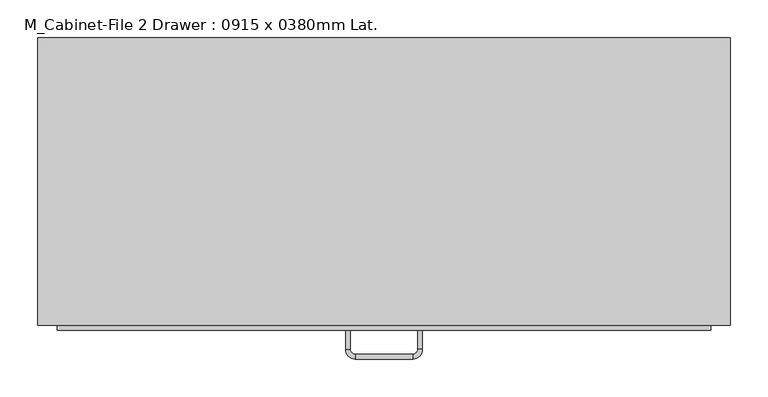
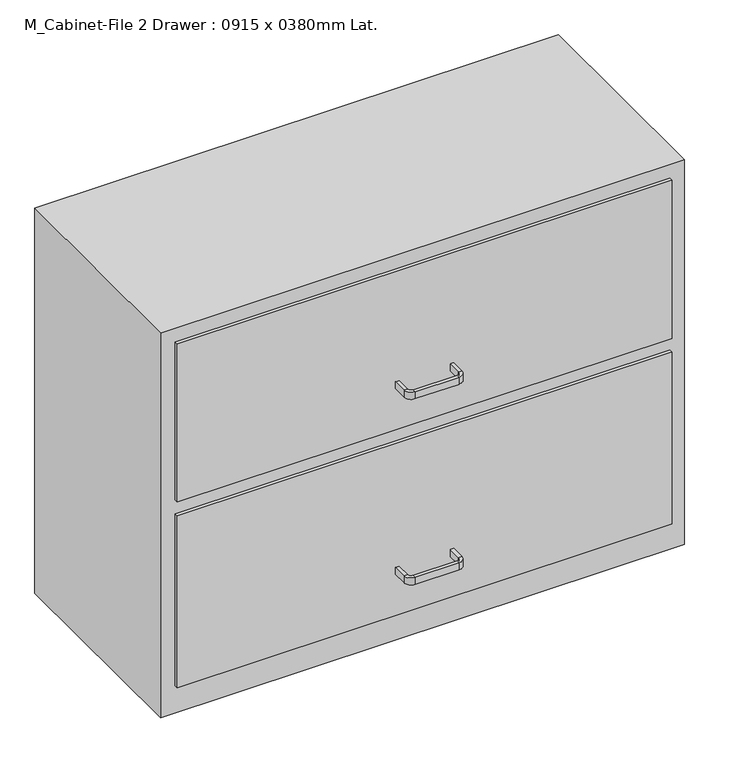
"""IFC4 building model written with IfcOpenShell, lengths in millimetres: furniture geometry, M_Cabinet-File 2 Drawer : 0915 x 0380mm Lat.."""

from ifc_helpers import new_model, si_unit, frame, origin, origin_with_axes, place, context, project, spatial, polyline, circle_curve, outline, extrude, source, transform, mapped, element, save
from ifc_brep_helpers import plane_surface, cylinder_surface, revolved_surface, advanced_brep


def m_cabinet_file_2_drawer_0915_x_0380mm_lat_9df0d5dd(model_context):
    return source(origin(), model_context, "Body", "SolidModel", [
        extrude(outline(polyline([(304.203553, -338.4843001), (-559.996447, -338.4843001), (-559.996447, -332.1343001), (304.203553, -332.1343001), (304.203553, -338.4843001)])), frame((0.0, 0.0, 393.7), z_axis=(0.0, 0.0, 1.0), x_axis=(1.0, 0.0, 0.0)), (0.0, 0.0, 1.0), 291.9),
        extrude(outline(polyline([(304.203553, -338.4843001), (-559.996447, -338.4843001), (-559.996447, -332.1343001), (304.203553, -332.1343001), (304.203553, -338.4843001)])), frame((0.0, 0.0, 50.8), z_axis=(0.0, 0.0, 1.0), x_axis=(1.0, 0.0, 0.0)), (0.0, 0.0, 1.0), 317.5),
        advanced_brep(
        [(-172.346447, -338.4843001, 127.0), (-178.696447, -338.4843001, 127.0), (-178.696447, -338.4843001, 139.7), (-172.346447, -338.4843001, 139.7), (-172.346447, -363.8843001, 127.0), (-178.696447, -363.8843001, 127.0), (-178.696447, -363.8843001, 139.7), (-172.346447, -363.8843001, 139.7), (-165.996447, -376.5843001, 127.0), (-165.996447, -370.2343001, 127.0), (-165.996447, -376.5843001, 139.7), (-165.996447, -370.2343001, 139.7), (-89.796447, -370.2343001, 127.0), (-89.796447, -376.5843001, 127.0), (-89.796447, -376.5843001, 139.7), (-89.796447, -370.2343001, 139.7), (-77.096447, -363.8843001, 127.0), (-83.446447, -363.8843001, 127.0), (-77.096447, -363.8843001, 139.7), (-83.446447, -363.8843001, 139.7), (-83.446447, -338.4843001, 127.0), (-83.446447, -338.4843001, 139.7), (-77.096447, -338.4843001, 139.7), (-77.096447, -338.4843001, 127.0)],
        [
            (0, 1),
            (1, 2),
            (2, 3),
            (3, 0),
            (0, 4),
            (4, 5),
            (5, 1),
            (5, 6),
            (6, 2),
            (6, 7),
            (7, 3),
            (7, 4),
            (8, 5, circle_curve(frame((-165.996447, -363.8843001, 127.0), z_axis=(0.0, 0.0, -1.0), x_axis=(-1.0, 0.0, 0.0)), 12.7)),
            (4, 9, circle_curve(frame((-165.996447, -363.8843001, 127.0), z_axis=(0.0, 0.0, 1.0), x_axis=(-1.0, 0.0, 0.0)), 6.35)),
            (9, 8),
            (10, 6, circle_curve(frame((-165.996447, -363.8843001, 139.7), z_axis=(0.0, 0.0, -1.0), x_axis=(-1.0, 0.0, 0.0)), 12.7)),
            (8, 10),
            (11, 7, circle_curve(frame((-165.996447, -363.8843001, 139.7), z_axis=(0.0, 0.0, -1.0), x_axis=(-1.0, 0.0, 0.0)), 6.35)),
            (10, 11),
            (11, 9),
            (9, 12),
            (12, 13),
            (13, 8),
            (13, 14),
            (14, 10),
            (14, 15),
            (15, 11),
            (15, 12),
            (16, 13, circle_curve(frame((-89.796447, -363.8843001, 127.0), z_axis=(0.0, 0.0, -1.0), x_axis=(0.0, -1.0, 0.0)), 12.7)),
            (12, 17, circle_curve(frame((-89.796447, -363.8843001, 127.0), z_axis=(0.0, 0.0, 1.0), x_axis=(0.0, -1.0, 0.0)), 6.35)),
            (17, 16),
            (18, 14, circle_curve(frame((-89.796447, -363.8843001, 139.7), z_axis=(0.0, 0.0, -1.0), x_axis=(0.0, -1.0, 0.0)), 12.7)),
            (16, 18),
            (19, 15, circle_curve(frame((-89.796447, -363.8843001, 139.7), z_axis=(0.0, 0.0, -1.0), x_axis=(0.0, -1.0, 0.0)), 6.35)),
            (18, 19),
            (19, 17),
            (20, 21),
            (21, 22),
            (22, 23),
            (23, 20),
            (17, 20),
            (23, 16),
            (22, 18),
            (21, 19),
        ],
        [
            plane_surface(frame((-661.3382215, -338.4843001, 0.0), z_axis=(0.0, 1.0, 0.0), x_axis=(0.0, 0.0, -1.0))),
            plane_surface(frame((-172.346447, -338.4843001, 127.0), z_axis=(0.0, 0.0, -1.0), x_axis=(0.0, -1.0, 0.0))),
            plane_surface(frame((-178.696447, -338.4843001, 127.0), z_axis=(-1.0, 0.0, 0.0), x_axis=(0.0, -1.0, 0.0))),
            plane_surface(frame((-178.696447, -338.4843001, 139.7), z_axis=(0.0, 0.0, 1.0), x_axis=(0.0, -1.0, 0.0))),
            plane_surface(frame((-172.346447, -338.4843001, 139.7), z_axis=(1.0, 0.0, 0.0), x_axis=(0.0, -1.0, 0.0))),
            plane_surface(frame((-165.996447, -363.8843001, 127.0), z_axis=(0.0, 0.0, -1.0), x_axis=(-1.0, 0.0, 0.0))),
            cylinder_surface(frame((-165.996447, -363.8843001, 0.0), z_axis=(0.0, 0.0, 1.0), x_axis=(-1.0, 0.0, 0.0)), 12.7),
            plane_surface(frame((-165.996447, -363.8843001, 139.7), z_axis=(0.0, 0.0, 1.0), x_axis=(-1.0, 0.0, 0.0))),
            revolved_surface(polyline([(-172.34644699999998, -363.8843001, 139.7), (-172.34644699999998, -363.8843001, 127.0)]), (-165.996447, -363.8843001, 0.0), (0.0, 0.0, 1.0)),
            plane_surface(frame((-165.996447, -370.2343001, 127.0), z_axis=(0.0, 0.0, -1.0), x_axis=(1.0, 0.0, 0.0))),
            plane_surface(frame((-165.996447, -376.5843001, 127.0), z_axis=(0.0, -1.0, 0.0), x_axis=(1.0, 0.0, 0.0))),
            plane_surface(frame((-165.996447, -376.5843001, 139.7), z_axis=(0.0, 0.0, 1.0), x_axis=(1.0, 0.0, 0.0))),
            plane_surface(frame((-165.996447, -370.2343001, 139.7), z_axis=(0.0, 1.0, 0.0), x_axis=(1.0, 0.0, 0.0))),
            plane_surface(frame((-89.796447, -363.8843001, 127.0), z_axis=(0.0, 0.0, -1.0), x_axis=(0.0, -1.0, 0.0))),
            cylinder_surface(frame((-89.796447, -363.8843001, 0.0), z_axis=(0.0, 0.0, 1.0), x_axis=(0.0, -1.0, 0.0)), 12.7),
            plane_surface(frame((-89.796447, -363.8843001, 139.7), z_axis=(0.0, 0.0, 1.0), x_axis=(0.0, -1.0, 0.0))),
            revolved_surface(polyline([(-89.796447, -370.23430010000004, 139.7), (-89.796447, -370.23430010000004, 127.0)]), (-89.796447, -363.8843001, 0.0), (0.0, 0.0, 1.0)),
            plane_surface(frame((-559.7382215, -338.4843001, 0.0), z_axis=(0.0, 1.0, 0.0), x_axis=(0.0, 0.0, 1.0))),
            plane_surface(frame((-83.446447, -363.8843001, 127.0), z_axis=(0.0, 0.0, -1.0), x_axis=(0.0, 1.0, 0.0))),
            plane_surface(frame((-77.096447, -363.8843001, 127.0), z_axis=(1.0, 0.0, 0.0), x_axis=(0.0, 1.0, 0.0))),
            plane_surface(frame((-77.096447, -363.8843001, 139.7), z_axis=(0.0, 0.0, 1.0), x_axis=(0.0, 1.0, 0.0))),
            plane_surface(frame((-83.446447, -363.8843001, 139.7), z_axis=(-1.0, 0.0, 0.0), x_axis=(0.0, 1.0, 0.0))),
        ],
        [
            (0, [[1, 2, 3, 4]]),
            (1, [[-1, 5, 6, 7]]),
            (2, [[-2, -7, 8, 9]]),
            (3, [[-3, -9, 10, 11]]),
            (4, [[-4, -11, 12, -5]]),
            (5, [[13, -6, 14, 15]]),
            (6, [[16, -8, -13, 17]]),
            (7, [[18, -10, -16, 19]]),
            (8, [[-14, -12, -18, 20]]),
            (9, [[-15, 21, 22, 23]]),
            (10, [[-17, -23, 24, 25]]),
            (11, [[-19, -25, 26, 27]]),
            (12, [[-20, -27, 28, -21]]),
            (13, [[29, -22, 30, 31]]),
            (14, [[32, -24, -29, 33]]),
            (15, [[34, -26, -32, 35]]),
            (16, [[-30, -28, -34, 36]]),
            (17, [[37, 38, 39, 40]]),
            (18, [[-31, 41, -40, 42]]),
            (19, [[-33, -42, -39, 43]]),
            (20, [[-35, -43, -38, 44]]),
            (21, [[-36, -44, -37, -41]]),
        ],
    ),
        advanced_brep(
        [(-172.346447, -338.4843001, 469.9), (-178.696447, -338.4843001, 469.9), (-178.696447, -338.4843001, 482.6), (-172.346447, -338.4843001, 482.6), (-172.346447, -363.8843001, 469.9), (-178.696447, -363.8843001, 469.9), (-178.696447, -363.8843001, 482.6), (-172.346447, -363.8843001, 482.6), (-165.996447, -376.5843001, 469.9), (-165.996447, -370.2343001, 469.9), (-165.996447, -376.5843001, 482.6), (-165.996447, -370.2343001, 482.6), (-89.796447, -370.2343001, 469.9), (-89.796447, -376.5843001, 469.9), (-89.796447, -376.5843001, 482.6), (-89.796447, -370.2343001, 482.6), (-77.096447, -363.8843001, 469.9), (-83.446447, -363.8843001, 469.9), (-77.096447, -363.8843001, 482.6), (-83.446447, -363.8843001, 482.6), (-83.446447, -338.4843001, 469.9), (-83.446447, -338.4843001, 482.6), (-77.096447, -338.4843001, 482.6), (-77.096447, -338.4843001, 469.9)],
        [
            (0, 1),
            (1, 2),
            (2, 3),
            (3, 0),
            (0, 4),
            (4, 5),
            (5, 1),
            (5, 6),
            (6, 2),
            (6, 7),
            (7, 3),
            (7, 4),
            (8, 5, circle_curve(frame((-165.996447, -363.8843001, 469.9), z_axis=(0.0, 0.0, -1.0), x_axis=(-1.0, 0.0, 0.0)), 12.7)),
            (4, 9, circle_curve(frame((-165.996447, -363.8843001, 469.9), z_axis=(0.0, 0.0, 1.0), x_axis=(-1.0, 0.0, 0.0)), 6.35)),
            (9, 8),
            (10, 6, circle_curve(frame((-165.996447, -363.8843001, 482.6), z_axis=(0.0, 0.0, -1.0), x_axis=(-1.0, 0.0, 0.0)), 12.7)),
            (8, 10),
            (11, 7, circle_curve(frame((-165.996447, -363.8843001, 482.6), z_axis=(0.0, 0.0, -1.0), x_axis=(-1.0, 0.0, 0.0)), 6.35)),
            (10, 11),
            (11, 9),
            (9, 12),
            (12, 13),
            (13, 8),
            (13, 14),
            (14, 10),
            (14, 15),
            (15, 11),
            (15, 12),
            (16, 13, circle_curve(frame((-89.796447, -363.8843001, 469.9), z_axis=(0.0, 0.0, -1.0), x_axis=(0.0, -1.0, 0.0)), 12.7)),
            (12, 17, circle_curve(frame((-89.796447, -363.8843001, 469.9), z_axis=(0.0, 0.0, 1.0), x_axis=(0.0, -1.0, 0.0)), 6.35)),
            (17, 16),
            (18, 14, circle_curve(frame((-89.796447, -363.8843001, 482.6), z_axis=(0.0, 0.0, -1.0), x_axis=(0.0, -1.0, 0.0)), 12.7)),
            (16, 18),
            (19, 15, circle_curve(frame((-89.796447, -363.8843001, 482.6), z_axis=(0.0, 0.0, -1.0), x_axis=(0.0, -1.0, 0.0)), 6.35)),
            (18, 19),
            (19, 17),
            (20, 21),
            (21, 22),
            (22, 23),
            (23, 20),
            (17, 20),
            (23, 16),
            (22, 18),
            (21, 19),
        ],
        [
            plane_surface(frame((-661.3382215, -338.4843001, 0.0), z_axis=(0.0, 1.0, 0.0), x_axis=(0.0, 0.0, -1.0))),
            plane_surface(frame((-172.346447, -338.4843001, 469.9), z_axis=(0.0, 0.0, -1.0), x_axis=(0.0, -1.0, 0.0))),
            plane_surface(frame((-178.696447, -338.4843001, 469.9), z_axis=(-1.0, 0.0, 0.0), x_axis=(0.0, -1.0, 0.0))),
            plane_surface(frame((-178.696447, -338.4843001, 482.6), z_axis=(0.0, 0.0, 1.0), x_axis=(0.0, -1.0, 0.0))),
            plane_surface(frame((-172.346447, -338.4843001, 482.6), z_axis=(1.0, 0.0, 0.0), x_axis=(0.0, -1.0, 0.0))),
            plane_surface(frame((-165.996447, -363.8843001, 469.9), z_axis=(0.0, 0.0, -1.0), x_axis=(-1.0, 0.0, 0.0))),
            cylinder_surface(frame((-165.996447, -363.8843001, 0.0), z_axis=(0.0, 0.0, 1.0), x_axis=(-1.0, 0.0, 0.0)), 12.7),
            plane_surface(frame((-165.996447, -363.8843001, 482.6), z_axis=(0.0, 0.0, 1.0), x_axis=(-1.0, 0.0, 0.0))),
            revolved_surface(polyline([(-172.34644699999998, -363.8843001, 482.6), (-172.34644699999998, -363.8843001, 469.9)]), (-165.996447, -363.8843001, 0.0), (0.0, 0.0, 1.0)),
            plane_surface(frame((-165.996447, -370.2343001, 469.9), z_axis=(0.0, 0.0, -1.0), x_axis=(1.0, 0.0, 0.0))),
            plane_surface(frame((-165.996447, -376.5843001, 469.9), z_axis=(0.0, -1.0, 0.0), x_axis=(1.0, 0.0, 0.0))),
            plane_surface(frame((-165.996447, -376.5843001, 482.6), z_axis=(0.0, 0.0, 1.0), x_axis=(1.0, 0.0, 0.0))),
            plane_surface(frame((-165.996447, -370.2343001, 482.6), z_axis=(0.0, 1.0, 0.0), x_axis=(1.0, 0.0, 0.0))),
            plane_surface(frame((-89.796447, -363.8843001, 469.9), z_axis=(0.0, 0.0, -1.0), x_axis=(0.0, -1.0, 0.0))),
            cylinder_surface(frame((-89.796447, -363.8843001, 0.0), z_axis=(0.0, 0.0, 1.0), x_axis=(0.0, -1.0, 0.0)), 12.7),
            plane_surface(frame((-89.796447, -363.8843001, 482.6), z_axis=(0.0, 0.0, 1.0), x_axis=(0.0, -1.0, 0.0))),
            revolved_surface(polyline([(-89.796447, -370.23430010000004, 482.6), (-89.796447, -370.23430010000004, 469.9)]), (-89.796447, -363.8843001, 0.0), (0.0, 0.0, 1.0)),
            plane_surface(frame((-559.7382215, -338.4843001, 0.0), z_axis=(0.0, 1.0, 0.0), x_axis=(0.0, 0.0, 1.0))),
            plane_surface(frame((-83.446447, -363.8843001, 469.9), z_axis=(0.0, 0.0, -1.0), x_axis=(0.0, 1.0, 0.0))),
            plane_surface(frame((-77.096447, -363.8843001, 469.9), z_axis=(1.0, 0.0, 0.0), x_axis=(0.0, 1.0, 0.0))),
            plane_surface(frame((-77.096447, -363.8843001, 482.6), z_axis=(0.0, 0.0, 1.0), x_axis=(0.0, 1.0, 0.0))),
            plane_surface(frame((-83.446447, -363.8843001, 482.6), z_axis=(-1.0, 0.0, 0.0), x_axis=(0.0, 1.0, 0.0))),
        ],
        [
            (0, [[1, 2, 3, 4]]),
            (1, [[-1, 5, 6, 7]]),
            (2, [[-2, -7, 8, 9]]),
            (3, [[-3, -9, 10, 11]]),
            (4, [[-4, -11, 12, -5]]),
            (5, [[13, -6, 14, 15]]),
            (6, [[16, -8, -13, 17]]),
            (7, [[18, -10, -16, 19]]),
            (8, [[-14, -12, -18, 20]]),
            (9, [[-15, 21, 22, 23]]),
            (10, [[-17, -23, 24, 25]]),
            (11, [[-19, -25, 26, 27]]),
            (12, [[-20, -27, 28, -21]]),
            (13, [[29, -22, 30, 31]]),
            (14, [[32, -24, -29, 33]]),
            (15, [[34, -26, -32, 35]]),
            (16, [[-30, -28, -34, 36]]),
            (17, [[37, 38, 39, 40]]),
            (18, [[-31, 41, -40, 42]]),
            (19, [[-33, -42, -39, 43]]),
            (20, [[-35, -43, -38, 44]]),
            (21, [[-36, -44, -37, -41]]),
        ],
    ),
        extrude(outline(polyline([(329.603553, 47.8656999), (329.603553, -332.1343001), (-585.396447, -332.1343001), (-585.396447, 47.8656999), (329.603553, 47.8656999)])), origin_with_axes(), (0.0, 0.0, 1.0), 711.0),
    ])


if __name__ == "__main__":
    model = new_model("IFC4")
    model_context = context("Model", 3, world=origin())
    ifc_project = project(units=[si_unit("LENGTHUNIT", "METRE", prefix="MILLI")], contexts=[model_context])
    site = spatial("IfcSite", under=ifc_project)
    building = spatial("IfcBuilding", under=site)
    placement = place(None, origin())
    m_cabinet_file_2_drawer_0915_x_0380mm_lat_shape = m_cabinet_file_2_drawer_0915_x_0380mm_lat_9df0d5dd(model_context)
    element("IfcFurniture", 1, ObjectType="M_Cabinet-File 2 Drawer : 0915 x 0380mm Lat.", at=placement, inside=building, context=model_context, shape_type="MappedRepresentation", body=[
        mapped(m_cabinet_file_2_drawer_0915_x_0380mm_lat_shape, transform((0.0, 0.0, 0.0), x_axis=(1.0, 0.0, 0.0), y_axis=(0.0, 1.0, 0.0), z_axis=(0.0, 0.0, 1.0))),
    ])
    save(model, "model.ifc")

# Revit data of these elements
# Type "M_Cabinet-File 2 Drawer : 0915 x 0380mm Lat."
#   Depth = 380 mm
#   Height = 711 mm
#   Width = 915 mm
#   Cabinet Material = Steel, Paint Finish, Ivory, Glossy
#   Handle Material = Steel, Chrome Plated
#   Default Elevation = 0
# Element 1 (IfcFurniture, "M_Cabinet-File 2 Drawer : 0915 x 0380mm Lat.")
#   Materials on its faces: "Steel, Chrome Plated", "Steel, Paint Finish, Ivory, Glossy"
# Materials
#   "Steel, Paint Finish, Ivory, Glossy": class "Metal", colour RGB 247 247 239, transparency 0, Description = "Steel, paint finish, ivory, glossy", Cost = 0
#   "Steel, Chrome Plated": class "Metal", colour RGB 244 244 244, transparency 0, Description = "Chromiuim plated steel", Cost = 0
